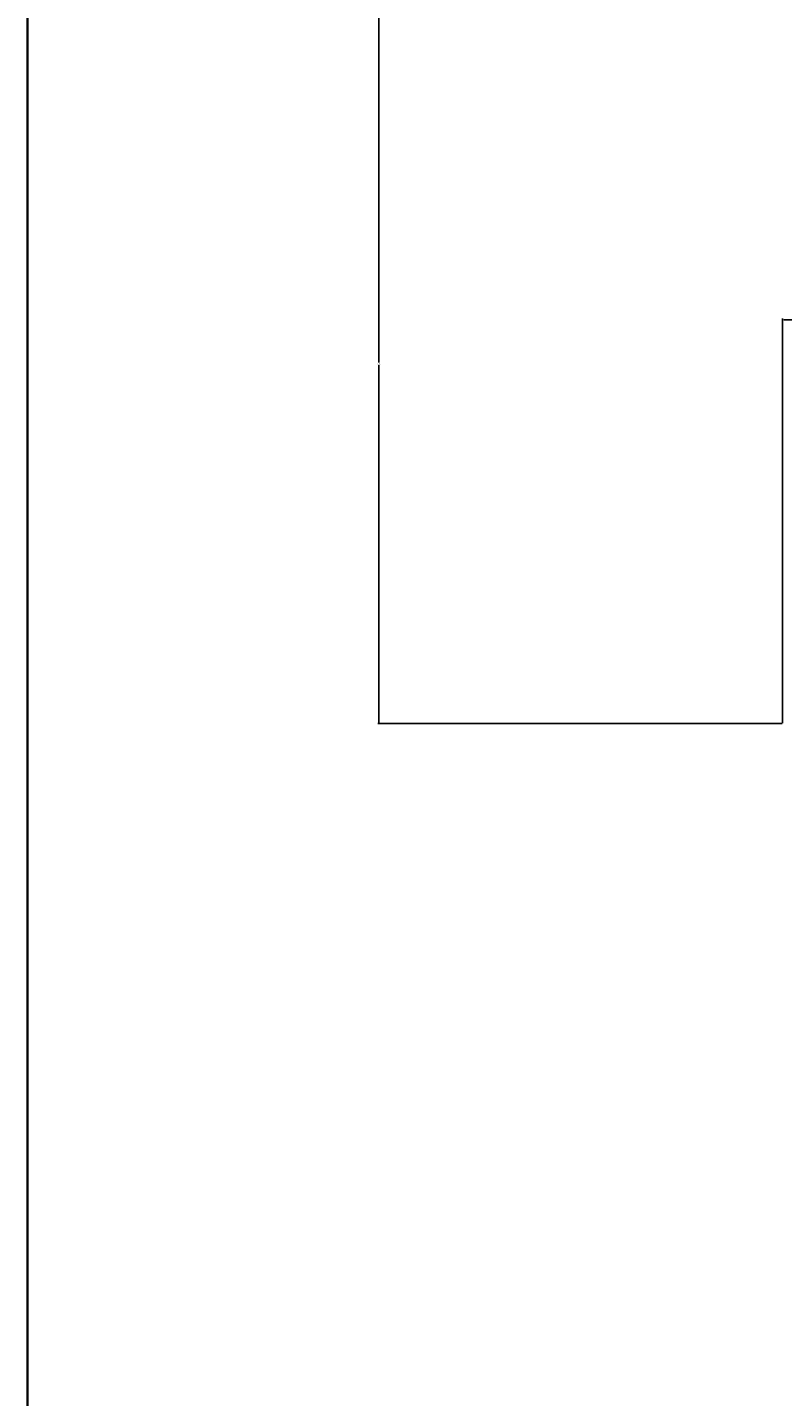
# Model space of a CAD drawing. Units: inches. Extents: x 1962 to 2771, y 1245 to 2660.
# Tile 22 of 114: x 1962 to 2072, y 1831 to 2030. Entities that reach past the tile are written whole.
import ezdxf

# ---------------------------------------------------------------- set-up
doc = ezdxf.new("R2010")
doc.units = ezdxf.units.IN
doc.layers.add('A-ANNO-DIMS', color=2, linetype='Continuous', lineweight=18)
doc.layers.add('A-ANNO-TTLB', color=7, linetype='Continuous', lineweight=35)
doc.styles.get("Standard").update_dxf_attribs({"font": 'arial.ttf'})
doc.dimstyles.get("Standard").update_dxf_attribs({"dimtxt": 0.18, "dimasz": 0.18, "dimexe": 0.18, "dimexo": 0.0625, "dimgap": 0.09, "dimtad": 0, "dimtih": 1, "dimtoh": 1, "dimdec": 4, "dimzin": 0, "dimdsep": 46, "dimtxsty": 'Standard', "dimcen": 0.09, "dimadec": 0, "dimazin": 0, "dimtfac": 1, "dimtdec": 4, "dimtofl": 0, "dimtmove": 0, "dimatfit": 3, "dimfxl": 1, "dimtolj": 1, "dimtzin": 0, "dimarcsym": 0})

# ---------------------------------------------------------------- blocks, each defined once
blk = doc.blocks.new('*D41')
at = {"layer": 'A-ANNO-DIMS', "color": 0, "lineweight": -2, "transparency": 16777216}
for p, q in [((2072.02, 1928.91), (2072.02, 1987.97)), ((2072.2, 1987.79), (2078.71, 1987.79)), ((2086.13, 1987.79), (2079.62, 1987.79)), ((2086.31, 1928.91), (2086.31, 1987.97))]:
    blk.add_line(p, q, dxfattribs=at)
at = {"layer": 'A-ANNO-DIMS', "color": 0, "transparency": 16777216}
for points in [[(2072.2, 1987.82), (2072.2, 1987.76), (2072.02, 1987.79)], [(2086.13, 1987.82), (2086.13, 1987.76), (2086.31, 1987.79)]]:
    blk.add_solid(points, dxfattribs=at)
at = {"layer": 'Defpoints', "color": 0, "transparency": 16777216}
for p in [(2086.31, 1987.79), (2072.02, 1928.84), (2086.31, 1928.84)]:
    blk.add_point(p, dxfattribs=at)
at = {"layer": 'A-ANNO-DIMS', "color": 0, "transparency": 16777216, "insert": (2079.16, 1987.79), "char_height": 0.18, "attachment_point": 5}
blk.add_mtext('\\A1;14.287', dxfattribs=at)
blk = doc.blocks.new('*D44')
at = {"layer": 'A-ANNO-DIMS', "color": 0, "lineweight": -2, "transparency": 16777216}
for p, q in [((2071.96, 2033.84), (2012.89, 2033.84)), ((2013.07, 2033.66), (2013.07, 1981.53)), ((2013.07, 1929.02), (2013.07, 1981.16)), ((2071.96, 1928.84), (2012.89, 1928.84))]:
    blk.add_line(p, q, dxfattribs=at)
at = {"layer": 'A-ANNO-DIMS', "color": 0, "transparency": 16777216}
for points in [[(2013.04, 2033.66), (2013.1, 2033.66), (2013.07, 2033.84)], [(2013.04, 1929.02), (2013.1, 1929.02), (2013.07, 1928.84)]]:
    blk.add_solid(points, dxfattribs=at)
at = {"layer": 'Defpoints', "color": 0, "transparency": 16777216}
for p in [(2072.02, 2033.84), (2013.07, 1928.84), (2072.02, 1928.84)]:
    blk.add_point(p, dxfattribs=at)
at = {"layer": 'A-ANNO-DIMS', "color": 0, "transparency": 16777216, "insert": (2013.07, 1981.34), "char_height": 0.18, "attachment_point": 5}
blk.add_mtext('\\A1;105', dxfattribs=at)

msp = doc.modelspace()

# ---------------------------------------------------------------- linework, layer by layer
at = {"layer": 'A-ANNO-TTLB'}
msp.add_lwpolyline([(1961.7365, 2660.2579), (2771.213, 2660.2579), (2771.213, 1244.5817), (1961.7365, 1244.5817)], close=True, dxfattribs=at)

# ---------------------------------------------------------------- dimensions: what is measured, and where the dimension line sits
at = {"layer": 'A-ANNO-DIMS'}
dim = msp.add_linear_dim(base=(2013.0704, 1928.8437), p1=(2072.0204, 2033.8437), p2=(2072.0204, 1928.8437), angle=90, dimstyle='Standard', override={"dimdec": 0, "dimlfac": 1, "dimrnd": 0, "dimzin": 0, "dimdsep": 46, "dimlunit": 2}, dxfattribs=at)
dim.commit()
dim.dimension.update_dxf_attribs({"geometry": '*D44', "text_midpoint": (2013.0704, 1981.3437)})
dim = msp.add_linear_dim(base=(2086.3074, 1987.7937), p1=(2072.0204, 1928.8437), p2=(2086.3074, 1928.8437), dimstyle='Standard', override={"dimdec": 3, "dimlfac": 1, "dimrnd": 0, "dimzin": 0, "dimdsep": 46, "dimlunit": 2}, dxfattribs=at)
dim.commit()
dim.dimension.update_dxf_attribs({"geometry": '*D41', "text_midpoint": (2079.1639, 1987.7937)})

doc.saveas('drawing.dxf')
